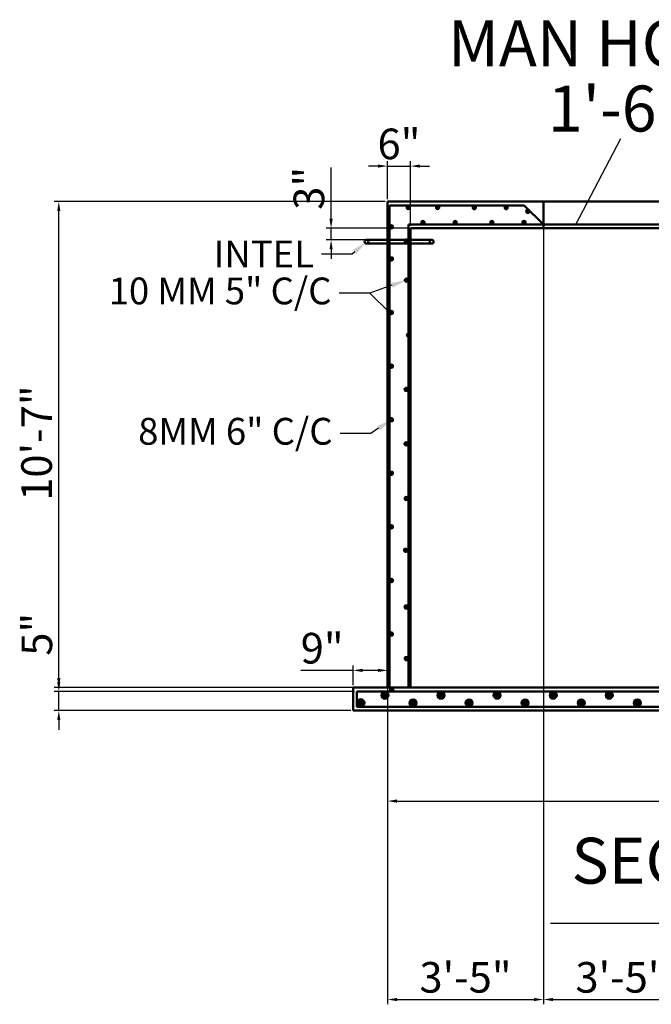
# Model space of a CAD drawing. Units: inches. Extents: x 2473 to 3272, y 1467 to 1853.
# Tile 1 of 3: x 2473 to 2638, y 1596 to 1853. Entities that reach past the tile are written whole.
import ezdxf
from ezdxf import colors
from ezdxf.entities.mleader import LeaderData, LeaderLine
from ezdxf.math import Vec2, Vec3

# ---------------------------------------------------------------- set-up
doc = ezdxf.new("R2010")
doc.units = ezdxf.units.IN
doc.header["$PDMODE"] = 36
for name, color, linetype, lineweight in [('S-ANNO-DIMS', 2, 'Continuous', 25), ('S-ANNO-TEXT', 7, 'Continuous', 25), ('S-CONC', 7, 'Continuous', 50), ('S-REIN', 3, 'Continuous', 35)]:
    doc.layers.add(name, color=color, linetype=linetype, lineweight=lineweight)
doc.styles.get("Standard").update_dxf_attribs({"font": '@Yu Gothic UI Semibold.ttf'})
doc.dimstyles.new('ISO-25', dxfattribs={"dimtxt": 8, "dimasz": 2.5, "dimexe": 1.25, "dimexo": 0.625, "dimtad": 1, "dimdec": 1, "dimlunit": 3, "dimtxsty": 'Standard', "dimcen": 2.5, "dimadec": 0, "dimazin": 0, "dimtfac": 1, "dimtdec": 1, "dimtmove": 0, "dimatfit": 3, "dimfxl": 1, "dimarcsym": 0})

# ---------------------------------------------------------------- blocks, each defined once
blk = doc.blocks.new('*D8')
at = {"layer": 'Defpoints', "color": 0, "transparency": 16777216}
for p in [(2569.47, 1678.69), (2773.47, 1678.69), (2773.47, 1649.05)]:
    blk.add_point(p, dxfattribs=at)
at = {"layer": 'S-ANNO-DIMS', "color": 0, "lineweight": -2, "transparency": 16777216}
for p, q in [((2569.47, 1678.06), (2569.47, 1647.8)), ((2773.47, 1678.06), (2773.47, 1647.8)), ((2571.97, 1649.05), (2770.97, 1649.05))]:
    blk.add_line(p, q, dxfattribs=at)
at = {"layer": 'S-ANNO-DIMS', "color": 0, "transparency": 16777216}
for points in [[(2571.97, 1649.47), (2571.97, 1648.63), (2569.47, 1649.05)], [(2770.97, 1649.47), (2770.97, 1648.63), (2773.47, 1649.05)]]:
    blk.add_solid(points, dxfattribs=at)
at = {"layer": 'S-ANNO-DIMS', "color": 0, "transparency": 16777216, "insert": (2671.47, 1653.76), "char_height": 8, "attachment_point": 5}
blk.add_mtext("17'", dxfattribs=at)
blk = doc.blocks.new('*D11')
at = {"layer": 'Defpoints', "color": 0, "transparency": 16777216}
for p in [(2483.5, 1677.69), (2561.47, 1677.69), (2560.47, 1672.69)]:
    blk.add_point(p, dxfattribs=at)
at = {"layer": 'S-ANNO-DIMS', "color": 0, "lineweight": -2, "transparency": 16777216}
for p, q in [((2483.5, 1680.19), (2483.5, 1698.01)), ((2560.84, 1677.69), (2482.25, 1677.69)), ((2483.5, 1672.69), (2483.5, 1677.69)), ((2559.84, 1672.69), (2482.25, 1672.69)), ((2483.5, 1670.19), (2483.5, 1667.69))]:
    blk.add_line(p, q, dxfattribs=at)
at = {"layer": 'S-ANNO-DIMS', "color": 0, "transparency": 16777216}
for points in [[(2483.08, 1680.19), (2483.91, 1680.19), (2483.5, 1677.69)], [(2483.08, 1670.19), (2483.91, 1670.19), (2483.5, 1672.69)]]:
    blk.add_solid(points, dxfattribs=at)
at = {"layer": 'S-ANNO-DIMS', "color": 0, "transparency": 16777216, "insert": (2478.8, 1692.63), "char_height": 8, "attachment_point": 5, "rotation": 90}
blk.add_mtext('5"', dxfattribs=at)
blk = doc.blocks.new('*D12')
at = {"layer": 'Defpoints', "color": 0, "transparency": 16777216}
for p in [(2560.47, 1683.19), (2560.47, 1678.69), (2569.47, 1678.69)]:
    blk.add_point(p, dxfattribs=at)
at = {"layer": 'S-ANNO-DIMS', "color": 0, "lineweight": -2, "transparency": 16777216}
for p, q in [((2560.47, 1683.19), (2546.8, 1683.19)), ((2560.47, 1679.31), (2560.47, 1684.44)), ((2566.97, 1683.19), (2562.97, 1683.19)), ((2569.47, 1679.31), (2569.47, 1684.44))]:
    blk.add_line(p, q, dxfattribs=at)
at = {"layer": 'S-ANNO-DIMS', "color": 0, "transparency": 16777216}
for points in [[(2562.97, 1683.61), (2562.97, 1682.77), (2560.47, 1683.19)], [(2566.97, 1683.61), (2566.97, 1682.77), (2569.47, 1683.19)]]:
    blk.add_solid(points, dxfattribs=at)
at = {"layer": 'S-ANNO-DIMS', "color": 0, "transparency": 16777216, "insert": (2552.38, 1687.95), "char_height": 8, "attachment_point": 5}
blk.add_mtext('9"', dxfattribs=at)
blk = doc.blocks.new('*D13')
at = {"layer": 'Defpoints', "color": 0, "transparency": 16777216}
for p in [(2483.5, 1805.69), (2569.47, 1805.69), (2569.47, 1678.69)]:
    blk.add_point(p, dxfattribs=at)
at = {"layer": 'S-ANNO-DIMS', "color": 0, "lineweight": -2, "transparency": 16777216}
for p, q in [((2568.84, 1805.69), (2482.25, 1805.69)), ((2483.5, 1681.19), (2483.5, 1803.19)), ((2568.84, 1678.69), (2482.25, 1678.69))]:
    blk.add_line(p, q, dxfattribs=at)
at = {"layer": 'S-ANNO-DIMS', "color": 0, "transparency": 16777216}
for points in [[(2483.08, 1803.19), (2483.91, 1803.19), (2483.5, 1805.69)], [(2483.08, 1681.19), (2483.91, 1681.19), (2483.5, 1678.69)]]:
    blk.add_solid(points, dxfattribs=at)
at = {"layer": 'S-ANNO-DIMS', "color": 0, "transparency": 16777216, "insert": (2478.72, 1742.58), "char_height": 8, "attachment_point": 5, "rotation": 90}
blk.add_mtext('10\'-7"', dxfattribs=at)
blk = doc.blocks.new('*D14')
at = {"layer": 'Defpoints', "color": 0, "transparency": 16777216}
for p in [(2575.47, 1814.95), (2569.47, 1805.69), (2575.47, 1798.69)]:
    blk.add_point(p, dxfattribs=at)
at = {"layer": 'S-ANNO-DIMS', "color": 0, "lineweight": -2, "transparency": 16777216}
for p, q in [((2569.47, 1806.31), (2569.47, 1816.2)), ((2575.47, 1799.31), (2575.47, 1816.2)), ((2566.97, 1814.95), (2564.47, 1814.95)), ((2569.47, 1814.95), (2575.47, 1814.95)), ((2577.97, 1814.95), (2580.47, 1814.95))]:
    blk.add_line(p, q, dxfattribs=at)
at = {"layer": 'S-ANNO-DIMS', "color": 0, "transparency": 16777216}
for points in [[(2566.97, 1815.36), (2566.97, 1814.53), (2569.47, 1814.95)], [(2577.97, 1815.36), (2577.97, 1814.53), (2575.47, 1814.95)]]:
    blk.add_solid(points, dxfattribs=at)
at = {"layer": 'S-ANNO-DIMS', "color": 0, "transparency": 16777216, "insert": (2572.47, 1819.71), "char_height": 8, "attachment_point": 5}
blk.add_mtext('6"', dxfattribs=at)
blk = doc.blocks.new('*D18')
at = {"layer": 'Defpoints', "color": 0, "transparency": 16777216}
for p in [(2554.71, 1798.69), (2575.47, 1798.69), (2569.47, 1795.69)]:
    blk.add_point(p, dxfattribs=at)
at = {"layer": 'S-ANNO-DIMS', "color": 0, "lineweight": -2, "transparency": 16777216}
for p, q in [((2554.71, 1801.19), (2554.71, 1814.61)), ((2574.84, 1798.69), (2553.46, 1798.69)), ((2554.71, 1795.69), (2554.71, 1798.69)), ((2568.84, 1795.69), (2553.46, 1795.69)), ((2554.71, 1793.19), (2554.71, 1790.69))]:
    blk.add_line(p, q, dxfattribs=at)
at = {"layer": 'S-ANNO-DIMS', "color": 0, "transparency": 16777216}
for points in [[(2554.29, 1801.19), (2555.12, 1801.19), (2554.71, 1798.69)], [(2554.29, 1793.19), (2555.12, 1793.19), (2554.71, 1795.69)]]:
    blk.add_solid(points, dxfattribs=at)
at = {"layer": 'S-ANNO-DIMS', "color": 0, "transparency": 16777216, "insert": (2549.95, 1809.15), "char_height": 8, "attachment_point": 5, "rotation": 90}
blk.add_mtext('3"', dxfattribs=at)
blk = doc.blocks.new('REBAR-SECTION-SMALL')
h = blk.add_hatch(color=256)
h.dxf.hatch_style = 1
h.paths.add_polyline_path([(2579.2, 1800.19, 1), (2578.2, 1800.19, 1)])
blk.add_circle((2578.7, 1800.19), 0.5)
blk = doc.blocks.new('REBAR-SECTION-LARGE')
h = blk.add_hatch(color=256)
h.dxf.hatch_style = 1
h.paths.add_polyline_path([(2652.73, 1800.68, 1), (2654.73, 1800.68, 1)])
blk.add_circle((2653.73, 1800.68), 1)
blk = doc.blocks.new('*D22')
at = {"layer": 'Defpoints', "color": 0, "transparency": 16777216}
for p in [(2569.47, 1805.69), (2610.27, 1805.69), (2610.27, 1597.2)]:
    blk.add_point(p, dxfattribs=at)
at = {"layer": 'S-ANNO-DIMS', "color": 0, "lineweight": -2, "transparency": 16777216}
for p, q in [((2569.47, 1805.06), (2569.47, 1595.95)), ((2610.27, 1805.06), (2610.27, 1595.95)), ((2571.97, 1597.2), (2607.77, 1597.2))]:
    blk.add_line(p, q, dxfattribs=at)
at = {"layer": 'S-ANNO-DIMS', "color": 0, "transparency": 16777216}
for points in [[(2571.97, 1597.61), (2571.97, 1596.78), (2569.47, 1597.2)], [(2607.77, 1597.61), (2607.77, 1596.78), (2610.27, 1597.2)]]:
    blk.add_solid(points, dxfattribs=at)
at = {"layer": 'S-ANNO-DIMS', "color": 0, "transparency": 16777216, "insert": (2589.87, 1601.96), "char_height": 8, "attachment_point": 5}
blk.add_mtext('3\'-5"', dxfattribs=at)
blk = doc.blocks.new('*D23')
at = {"layer": 'Defpoints', "color": 0, "transparency": 16777216}
for p in [(2610.27, 1805.69), (2651.07, 1805.69), (2651.07, 1597.2)]:
    blk.add_point(p, dxfattribs=at)
at = {"layer": 'S-ANNO-DIMS', "color": 0, "lineweight": -2, "transparency": 16777216}
for p, q in [((2610.27, 1805.06), (2610.27, 1595.95)), ((2651.07, 1805.06), (2651.07, 1595.95)), ((2612.77, 1597.2), (2648.57, 1597.2))]:
    blk.add_line(p, q, dxfattribs=at)
at = {"layer": 'S-ANNO-DIMS', "color": 0, "transparency": 16777216}
for points in [[(2612.77, 1597.61), (2612.77, 1596.78), (2610.27, 1597.2)], [(2648.57, 1597.61), (2648.57, 1596.78), (2651.07, 1597.2)]]:
    blk.add_solid(points, dxfattribs=at)
at = {"layer": 'S-ANNO-DIMS', "color": 0, "transparency": 16777216, "insert": (2630.67, 1601.96), "char_height": 8, "attachment_point": 5}
blk.add_mtext('3\'-5"', dxfattribs=at)

msp = doc.modelspace()

# ---------------------------------------------------------------- linework, layer by layer
at = {"layer": 'S-ANNO-TEXT'}
for p, q in [((2618.71, 1799.69), (2630.53, 1822.12)), ((2569.97, 1776.69), (2564.82, 1781.75)), ((2612.08, 1617.15), (2728.34, 1617.15))]:
    msp.add_line(p, q, dxfattribs=at)
at = {"layer": 'S-CONC'}
for p, q in [((2569.47, 1805.69), (2773.47, 1805.69)), ((2569.47, 1805.69), (2569.47, 1678.69)), ((2569.97, 1804.69), (2605.2, 1804.69)), ((2569.97, 1804.69), (2569.97, 1678.69)), ((2610.27, 1799.69), (2605.2, 1804.69)), ((2610.27, 1798.69), (2610.27, 1805.69)), ((2574.97, 1799.69), (2574.97, 1678.69)), ((2574.97, 1799.69), (2767.97, 1799.69)), ((2575.47, 1798.69), (2767.47, 1798.69)), ((2575.47, 1798.69), (2575.47, 1678.69)), ((2569.47, 1795.69), (2563.96, 1795.69)), ((2569.47, 1795.69), (2581.02, 1795.69)), ((2563.96, 1794.69), (2581.02, 1794.69)), ((2560.47, 1678.69), (2782.47, 1678.69)), ((2560.47, 1678.69), (2560.47, 1672.69)), ((2561.47, 1677.69), (2781.47, 1677.69)), ((2561.47, 1677.69), (2561.47, 1673.69)), ((2560.47, 1672.69), (2782.47, 1672.69)), ((2561.47, 1673.69), (2781.47, 1673.69))]:
    msp.add_line(p, q, dxfattribs=at)
for centre in [(2563.96, 1795.19), (2581.02, 1795.19)]:
    msp.add_circle(centre, 0.5, dxfattribs=at)

# ---------------------------------------------------------------- block references
at = {"layer": 'S-REIN', "rotation": 180}
for name, p in [('REBAR-SECTION-SMALL', (5153.61, 3604.31)), ('REBAR-SECTION-SMALL', (5161.27, 3604.31)), ('REBAR-SECTION-SMALL', (5170.87, 3604.3)), ('REBAR-SECTION-SMALL', (5179.2, 3604.3)), ('REBAR-SECTION-SMALL', (5184.87, 3603.32)), ('REBAR-SECTION-SMALL', (5149.17, 3599.26)), ('REBAR-SECTION-SMALL', (5157.43, 3600.38)), ('REBAR-SECTION-SMALL', (5165.86, 3600.38)), ('REBAR-SECTION-SMALL', (5175.44, 3600.38)), ('REBAR-SECTION-SMALL', (5183.87, 3600.38)), ('REBAR-SECTION-SMALL', (5153.07, 3595.56)), ('REBAR-SECTION-SMALL', (5149.17, 3590.88)), ('REBAR-SECTION-SMALL', (5153.1, 3585.32)), ('REBAR-SECTION-SMALL', (5149.17, 3576.88)), ('REBAR-SECTION-SMALL', (5153.67, 3570.98)), ('REBAR-SECTION-SMALL', (5149.17, 3562.88)), ('REBAR-SECTION-SMALL', (5153.06, 3556.8)), ('REBAR-SECTION-SMALL', (5149.17, 3548.88)), ('REBAR-SECTION-SMALL', (5153.01, 3542.59)), ('REBAR-SECTION-SMALL', (5149.17, 3534.88)), ('REBAR-SECTION-SMALL', (5153.07, 3528.3)), ('REBAR-SECTION-SMALL', (5149.17, 3520.88)), ('REBAR-SECTION-SMALL', (5152.9, 3514.76)), ('REBAR-SECTION-SMALL', (5149.17, 3506.88)), ('REBAR-SECTION-SMALL', (5153.03, 3499.94)), ('REBAR-SECTION-SMALL', (5149.17, 3492.88)), ('REBAR-SECTION-SMALL', (5153.09, 3486.45)), ('REBAR-SECTION-LARGE', (5222.53, 3477.37)), ('REBAR-SECTION-SMALL', (5149.25, 3478.41)), ('REBAR-SECTION-LARGE', (5237.19, 3477.37)), ('REBAR-SECTION-LARGE', (5251.86, 3477.37)), ('REBAR-SECTION-LARGE', (5266.53, 3477.37)), ('REBAR-SECTION-LARGE', (5281.19, 3477.37)), ('REBAR-SECTION-LARGE', (5216.25, 3475.42)), ('REBAR-SECTION-LARGE', (5229.86, 3475.37)), ('REBAR-SECTION-LARGE', (5244.53, 3475.37)), ('REBAR-SECTION-LARGE', (5259.19, 3475.37)), ('REBAR-SECTION-LARGE', (5273.86, 3475.37)), ('REBAR-SECTION-LARGE', (5288.53, 3475.37))]:
    msp.add_blockref(name, p, dxfattribs=at)

# ---------------------------------------------------------------- texts
at = {"layer": 'S-ANNO-TEXT'}
for s, p in [('MAN HOLE COVERS', (2585.29, 1840.99)), ('1\'-6"X1\'-6"', (2611.42, 1823.98)), ("SECTION 'A A'", (2617.57, 1627.47))]:
    msp.add_text(s, height=12, dxfattribs=at).set_placement(p)

# ---------------------------------------------------------------- dimensions: what is measured, and where the dimension line sits
at = {"layer": 'S-ANNO-DIMS'}
for base, p1, p2, picture, middle in [((2575.47, 1814.95), (2569.47, 1805.69), (2575.47, 1798.69), '*D14', (2572.47, 1814.95)), ((2773.47, 1649.05), (2569.47, 1678.69), (2773.47, 1678.69), '*D8', (2671.47, 1649.05))]:
    dim = msp.add_linear_dim(base=base, p1=p1, p2=p2, dimstyle='ISO-25', override={"dimclrd": 0, "dimclre": 0, "dimclrt": 0}, dxfattribs=at)
    dim.commit()
    dim.dimension.update_dxf_attribs({"geometry": picture, "text_midpoint": middle, "dimtype": 160})
dim = msp.add_linear_dim(base=(2554.71, 1798.69), p1=(2569.47, 1795.69), p2=(2575.47, 1798.69), angle=270, dimstyle='ISO-25', override={"dimclrd": 0, "dimclre": 0, "dimclrt": 0}, dxfattribs=at)
dim.commit()
dim.dimension.update_dxf_attribs({"geometry": '*D18', "text_midpoint": (2549.95, 1809.15)})
for base, p1, p2, angle, picture, middle in [((2483.5, 1805.69), (2569.47, 1678.69), (2569.47, 1805.69), 90, '*D13', (2483.5, 1742.58)), ((2483.5, 1677.69), (2560.47, 1672.69), (2561.47, 1677.69), 270, '*D11', (2483.5, 1692.63))]:
    dim = msp.add_linear_dim(base=base, p1=p1, p2=p2, angle=angle, dimstyle='ISO-25', override={"dimclrd": 0, "dimclre": 0, "dimclrt": 0}, dxfattribs=at)
    dim.commit()
    dim.dimension.update_dxf_attribs({"geometry": picture, "text_midpoint": middle, "dimtype": 160})
for base, p1, p2, override, picture, middle in [((2610.27, 1597.2), (2569.47, 1805.69), (2610.27, 1805.69), {"dimdec": 1, "dimlfac": 1, "dimrnd": 0, "dimzin": 1, "dimdsep": 46, "dimlunit": 4, "dimfrac": 2}, '*D22', (2589.87, 1601.96)), ((2651.07, 1597.2), (2610.27, 1805.69), (2651.07, 1805.69), {"dimdec": 1, "dimlfac": 1, "dimrnd": 0, "dimzin": 1, "dimdsep": 46, "dimlunit": 4, "dimfrac": 2}, '*D23', (2630.67, 1601.96)), ((2560.47, 1683.19), (2569.47, 1678.69), (2560.47, 1678.69), {"dimclrd": 0, "dimclre": 0, "dimclrt": 0}, '*D12', (2552.38, 1687.95))]:
    dim = msp.add_linear_dim(base=base, p1=p1, p2=p2, dimstyle='ISO-25', override=override, dxfattribs=at)
    dim.commit()
    dim.dimension.update_dxf_attribs({"geometry": picture, "text_midpoint": middle})

# ---------------------------------------------------------------- leaders
at = {"layer": 'S-ANNO-TEXT'}
ml = msp.add_multileader_mtext('Standard', dxfattribs=at)
ml.set_content('INTEL', color=256)
ml.set_leader_properties()
ml.build(insert=Vec2(0, 0))
ctx = ml.context
ctx.base_point, ctx.char_height, ctx.plane_origin = Vec3(2523.09, 1791.98), 7, Vec3(2563.96, 1795.19)
ctx.text_align_type = 2
notes = []
notes.append((ctx, [(0, (1, 1, 0), (2560.24, 1791.98), (-1, 0), 8, [(0, [(2563.96, 1795.19)], 0, [])])]))
ctx.mtext.insert, ctx.mtext.alignment, ctx.mtext.flow_direction = Vec3(2550.24, 1795.48), 3, 5
ml = msp.add_multileader_mtext('Standard', dxfattribs=at)
ml.set_content('10 MM 5" C/C', color=256)
ml.set_leader_properties()
ml.build(insert=Vec2(0, 0))
ctx = ml.context
ctx.base_point, ctx.char_height, ctx.plane_origin = Vec3(2490.91, 1781.75), 7, Vec3(2574.4, 1785.13)
ctx.text_align_type = 2
notes.append((ctx, [(0, (1, 1, 0), (2564.82, 1781.75), (-1, 0), 8, [(0, [(2574.4, 1785.13)], 0, [])])]))
ctx.mtext.insert, ctx.mtext.alignment, ctx.mtext.flow_direction = Vec3(2554.82, 1785.83), 3, 5
ml = msp.add_multileader_mtext('Standard', dxfattribs=at)
ml.set_content('8MM 6" C/C', color=256)
ml.set_leader_properties()
ml.build(insert=Vec2(0, 0))
ctx = ml.context
ctx.base_point, ctx.char_height, ctx.plane_origin = Vec3(2497.98, 1745.08), 7, Vec3(2570.47, 1748.69)
ctx.text_align_type = 2
notes.append((ctx, [(0, (1, 1, 0), (2565.1, 1745.08), (-1, 0), 8, [(0, [(2570.47, 1748.69)], 0, [])])]))
ctx.mtext.insert, ctx.mtext.alignment, ctx.mtext.flow_direction = Vec3(2555.1, 1749.16), 3, 5
for ctx, leaders in notes:
    for number, flags, end, landing, length, lines in leaders:
        leader = LeaderData()
        leader.index, (leader.has_last_leader_line, leader.has_dogleg_vector, leader.attachment_direction) = number, flags
        leader.last_leader_point, leader.dogleg_vector, leader.dogleg_length = Vec3(end), Vec3(landing), length
        for number, points, colour, breaks in lines:
            line = LeaderLine()
            line.index, line.vertices, line.color, line.breaks = number, Vec3.list(points), colors.encode_raw_color(colour), breaks
            leader.lines.append(line)
        ctx.leaders.append(leader)

doc.saveas('drawing.dxf')
